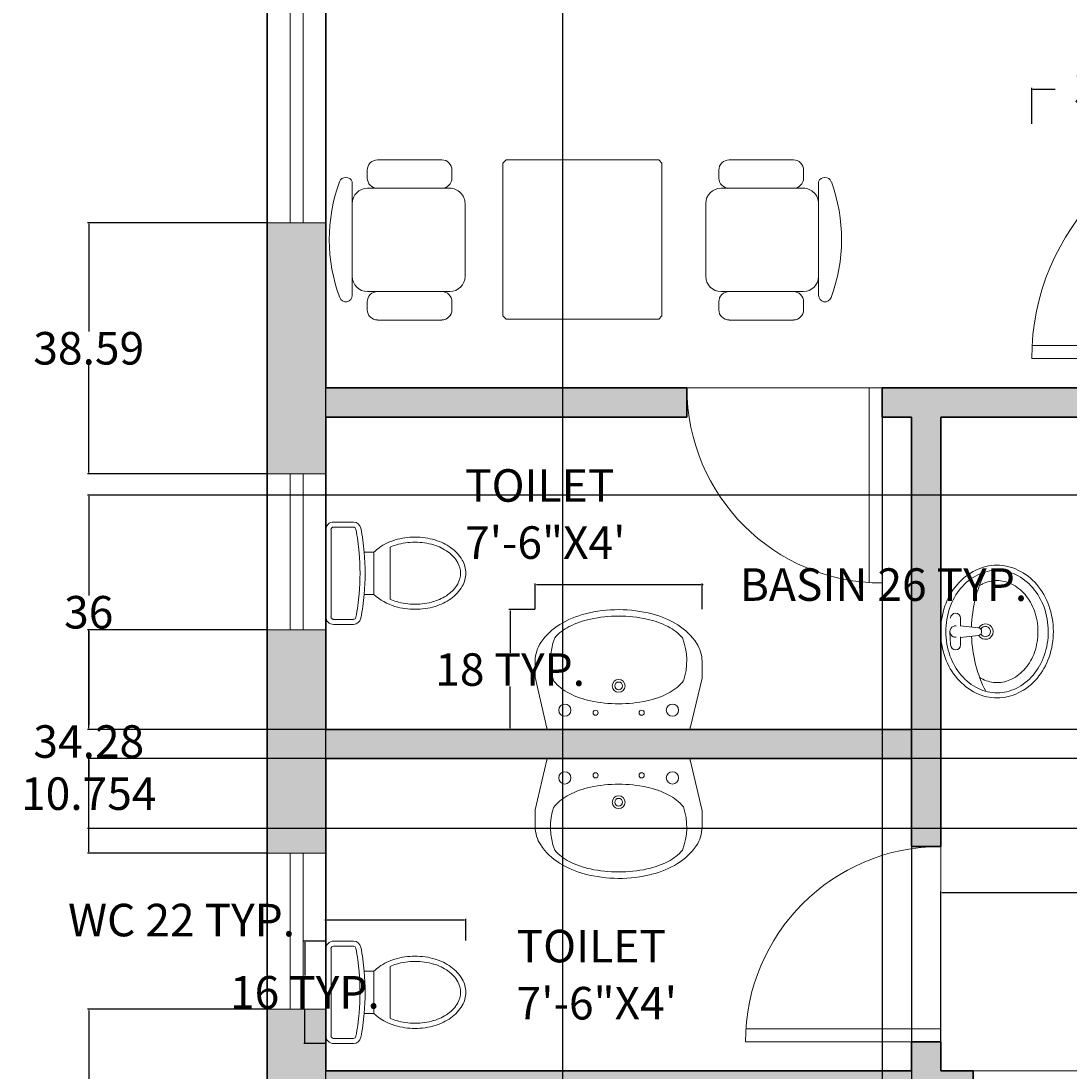
# Model space of a CAD drawing. Units: inches. Extents: x 2807 to 3326, y 2005 to 2580.
# Tile 8 of 12: x 2807 to 2968, y 2280 to 2441. Entities that reach past the tile are written whole.
import ezdxf

# ---------------------------------------------------------------- set-up
doc = ezdxf.new("R2010")
doc.units = ezdxf.units.IN
doc.header["$LTSCALE"] = 0.4
for name, color, linetype, lineweight in [('A-ANNO-DIMS', 2, 'Continuous', 18), ('A-AREA-IDEN', 5, 'Continuous', 18), ('A-FLOR-FIXT', 8, 'Continuous', 18), ('A-WALL-PATT', 231, 'Continuous', 13), ('DOORS', 144, 'Continuous', 18), ('Furniture', 7, 'Continuous', 15), ('WALL', 233, 'Continuous', 35), ('WINDOWS', 132, 'Continuous', 18)]:
    doc.layers.add(name, color=color, linetype=linetype, lineweight=lineweight)
doc.styles.get("Standard").update_dxf_attribs({"font": 'txt', "height": 5})
doc.dimstyles.get("Standard").update_dxf_attribs({"dimtxt": 0.18, "dimasz": 0.18, "dimexe": 0.18, "dimexo": 0.0625, "dimgap": 0.09, "dimtad": 0, "dimtih": 1, "dimtoh": 1, "dimdec": 4, "dimzin": 0, "dimdsep": 46, "dimtxsty": 'Standard', "dimcen": 0.09, "dimadec": 0, "dimazin": 0, "dimtfac": 1, "dimtdec": 4, "dimtofl": 0, "dimtmove": 0, "dimatfit": 3, "dimfxl": 1, "dimtolj": 1, "dimtzin": 0, "dimarcsym": 0})

# ---------------------------------------------------------------- blocks, each defined once
blk = doc.blocks.new('WIN-36')
at = {"ltscale": 0.4}
for p, q in [((0, 36), (0, 0)), ((9, 36), (0, 36)), ((3.5, 36), (3.5, 0)), ((5.5, 36), (5.5, 0)), ((9, 0), (9, 36)), ((0, 0), (9, 0))]:
    blk.add_line(p, q, dxfattribs=at)
blk = doc.blocks.new('WIN-24')
at = {"ltscale": 0.4}
for p, q in [((0, 0), (-9, 0)), ((-9, 0), (-9, -24)), ((-5.5, -24), (-5.5, 0)), ((-3.5, -24), (-3.5, 0)), ((0, -24), (0, 0)), ((-9, -24), (0, -24))]:
    blk.add_line(p, q, dxfattribs=at)
blk = doc.blocks.new('DOOR-30')
for p, q in [((0, 0), (-30, 0)), ((-2, -29.93), (-2, 0)), ((0, -30), (0, 0))]:
    blk.add_line(p, q)
blk.add_arc((0, 0), 30, 180, 270)
blk = doc.blocks.new('DOOR-36')
for p, q in [((0, 0), (-36, 0)), ((-2, -35.94), (-2, 0)), ((0, -36), (0, 0))]:
    blk.add_line(p, q)
blk.add_arc((0, 0), 36, 180, 270)
blk = doc.blocks.new('TABLE-SET-TWO')
for p, q in [((-7.94, 35.84), (-8.53, 35.84)), ((8.92, 35.84), (-7.94, 35.84)), ((-5.59, 35.84), (5.59, 35.84)), ((-10.73, 33.54), (-9.51, 33.54)), ((-7.94, 20.85), (-7.94, 33.49)), ((7.94, 33.49), (7.94, 20.85)), ((9.51, 33.54), (10.73, 33.54)), ((-12.31, 22.08), (-12.31, 31.97)), ((-7.94, 31.97), (-7.94, 22.08)), ((7.94, 22.08), (7.94, 31.97)), ((12.31, 31.97), (12.31, 22.08)), ((-9.51, 20.51), (-10.73, 20.51)), ((10.73, 20.51), (9.51, 20.51)), ((5.59, 18.5), (-5.59, 18.5)), ((-12.17, 12.19), (-11.66, 12.7)), ((-12.17, -11.26), (-12.17, 12.19)), ((-11.66, 12.7), (11.79, 12.7)), ((11.79, 12.7), (12.3, 12.19)), ((12.3, 12.19), (12.3, -11.26)), ((-11.66, -11.77), (-12.17, -11.26)), ((12.3, -11.26), (11.79, -11.77)), ((11.79, -11.77), (-11.66, -11.77)), ((5.59, -18.5), (-5.59, -18.5)), ((-9.51, -20.51), (-10.73, -20.51)), ((-7.94, -20.85), (-7.94, -33.49)), ((7.94, -33.49), (7.94, -20.85)), ((10.73, -20.51), (9.51, -20.51)), ((-12.31, -22.08), (-12.31, -31.97)), ((-7.94, -31.97), (-7.94, -22.08)), ((7.94, -22.08), (7.94, -31.97)), ((12.31, -31.97), (12.31, -22.08)), ((-10.73, -33.54), (-9.51, -33.54)), ((9.51, -33.54), (10.73, -33.54)), ((-7.94, -35.84), (-8.53, -35.84)), ((8.92, -35.84), (-7.94, -35.84)), ((-5.59, -35.84), (5.59, -35.84))]:
    blk.add_line(p, q)
for centre, radius, start, end in [((0.09, 13.6), 25.77, 69.9544, 110.3611), ((-8.53, 36.83), 0.986, 110.3611, 270), ((8.57, 36.82), 1.04, 290.0456, 69.9544), ((-5.59, 33.49), 2.35, 90, 180), ((5.59, 33.49), 2.35, 0, 90), ((-10.73, 31.97), 1.57, 90, 180), ((-9.51, 31.97), 1.57, 0, 90), ((9.51, 31.97), 1.57, 90, 180), ((10.73, 31.97), 1.57, 0, 90), ((-10.73, 22.08), 1.57, 180, 270), ((-9.51, 22.08), 1.57, 270, 0), ((9.51, 22.08), 1.57, 180, 270), ((10.73, 22.08), 1.57, 270, 0), ((-5.59, 20.85), 2.35, 180, 270), ((5.59, 20.85), 2.35, 270, 0), ((-5.59, -20.85), 2.35, 90, 180), ((5.59, -20.85), 2.35, 0, 90), ((-10.73, -22.08), 1.57, 90, 180), ((-9.51, -22.08), 1.57, 0, 90), ((9.51, -22.08), 1.57, 90, 180), ((10.73, -22.08), 1.57, 0, 90), ((-10.73, -31.97), 1.57, 180, 270), ((-9.51, -31.97), 1.57, 270, 0), ((9.51, -31.97), 1.57, 180, 270), ((10.73, -31.97), 1.57, 270, 0), ((-5.59, -33.49), 2.35, 180, 270), ((5.59, -33.49), 2.35, 270, 0), ((-8.53, -36.83), 0.986, 90, 249.6389), ((8.57, -36.82), 1.04, 290.0456, 69.9544), ((0.09, -13.6), 25.77, 249.6389, 290.0456)]:
    blk.add_arc(centre, radius, start, end)
blk = doc.blocks.new('WC')
for p, q in [((-1.18, 7.87), (-4.23, 7.87)), ((-1.18, 7.09), (-4.23, 7.09)), ((-0.79, -6.69), (-0.79, 6.69)), ((0, -6.69), (0, 6.69)), ((-9.87, -3.98), (-9.87, 3.98)), ((-7.37, -3.23), (-7.37, 3.26)), ((-7.37, 3.26), (-5.9, 3.26)), ((-7.37, -3.23), (-5.9, -3.23)), ((-4.23, -7.09), (-1.18, -7.09)), ((-4.23, -7.87), (-1.18, -7.87))]:
    blk.add_line(p, q)
for centre, radius, start, end in [((31.04, 0), 37.08, 169.2553, 174.96), ((-4.23, 6.69), 1.18, 90, 169.2553), ((31.04, 0), 36.29, 169.2553, 174.96), ((-4.23, 6.69), 0.394, 90, 169.2553), ((-1.18, 6.69), 1.18, 0, 90), ((-1.18, 6.69), 0.394, 0, 90), ((-14.49, -2.74), 8.17, 106.4045, 125.4032), ((-13.7, -5.39), 10.94, 90, 106.4045), ((-13.7, -5.39), 10.94, 73.5955, 90), ((-12.92, -2.74), 8.17, 47.2276, 73.5955), ((-15.68, -1.06), 6.11, 125.4032, 149.7669), ((-15.68, -1.06), 5.33, 125.4032, 149.7669), ((-14.49, -2.74), 7.39, 106.4045, 125.4032), ((-13.7, -5.39), 10.15, 90, 106.4045), ((-13.7, -5.39), 10.15, 73.5955, 90), ((-12.92, -2.74), 7.39, 65.5529, 73.5955), ((31.04, 0), 37.08, 174.96, 184.9899), ((-17.5, 0), 4, 149.7669, 180), ((-17.5, 0), 3.21, 149.7669, 180), ((31.04, 0), 36.29, 174.96, 184.9899), ((-17.5, 0), 4, 180, 210.2331), ((-17.5, 0), 3.21, 180, 210.2331), ((-15.68, 1.06), 6.11, 210.2331, 234.5968), ((-15.68, 1.06), 5.33, 210.2331, 234.5968), ((-11.73, 1.06), 6.11, 305.4032, 315.4553), ((31.04, 0), 37.08, 184.9899, 190.7447), ((31.04, 0), 36.29, 184.9899, 190.7447), ((-14.49, 2.74), 8.17, 234.5968, 253.5955), ((-14.49, 2.74), 7.39, 234.5968, 253.5955), ((-13.7, 5.39), 10.15, 253.5955, 270), ((-13.7, 5.39), 10.15, 270, 286.4045), ((-12.92, 2.74), 7.39, 286.4045, 294.4471), ((-12.92, 2.74), 8.17, 286.4045, 305.4032), ((-13.7, 5.39), 10.94, 253.5955, 270), ((-13.7, 5.39), 10.94, 270, 286.4045), ((-4.23, -6.69), 1.18, 190.7447, 270), ((-4.23, -6.69), 0.394, 190.7447, 270), ((-1.18, -6.69), 0.394, 270, 0), ((-1.18, -6.69), 1.18, 270, 0)]:
    blk.add_arc(centre, radius, start, end)
blk = doc.blocks.new('LAVATORY-WALL')
for p, q in [((-12.82, 8.02), (-12.82, 10.56)), ((12.82, 8.02), (12.82, 10.56)), ((-12.82, 8.02), (-11.02, 0.2)), ((9.76, 7.2), (9.85, 7.28)), ((9.86, 7.44), (9.86, 7.31)), ((12.82, 7.85), (11.02, 0.2)), ((-11.02, 0), (-11.02, 0.39)), ((11.02, 0), (-11.02, 0)), ((11.02, 0.39), (11.02, 0))]:
    blk.add_line(p, q)
for centre, radius in [((0, 6.69), 0.984), ((0, 6.69), 0.591), ((-8.27, 2.95), 0.945), ((8.27, 2.95), 0.945), ((8.27, 2.95), 0.945), ((8.27, 2.95), 0.945), ((-3.54, 2.56), 0.394), ((3.54, 2.56), 0.394)]:
    blk.add_circle(centre, radius)
for centre, radius, start, end in [((-1.65, 3.98), 14.22, 104.0583, 121.3573), ((-0.05, -2.38), 20.78, 89.7676, 104.0583), ((-0.05, -2.38), 20.78, 75.477, 89.7676), ((-1.62, 4.13), 13.11, 102.0046, 117.1742), ((0, -3.48), 20.89, 90, 102.0046), ((0, -3.48), 20.89, 77.9954, 90), ((1.62, 4.13), 13.11, 62.8258, 77.9954), ((1.59, 3.97), 14.22, 58.1779, 75.477), ((-4.1, 8.01), 9.5, 121.3573, 145.8048), ((-4.07, 8.92), 7.73, 117.1742, 138.1444), ((4.07, 8.92), 7.73, 41.9499, 62.8258), ((4.08, 7.98), 9.5, 33.7305, 58.1779), ((-7.83, 10.54), 4.99, 145.8048, 179.7676), ((-0.53, 10.56), 9.94, 159.3022, 198.4613), ((0.53, 10.56), 9.94, 341.5387, 20.6978), ((7.83, 10.48), 4.99, 359.7676, 33.7305), ((-7.83, 10.54), 4.99, 179.7676, 180.9606), ((-4.07, 12.42), 7.73, 220.3901, 242.8258), ((4.07, 12.42), 7.73, 297.1742, 318.6261), ((9.82, 7.31), 0.0394, 311.3224, 0), ((7.83, 8.04), 4.99, 357.883, 359.7676), ((-1.62, 17.21), 13.11, 242.8258, 257.9954), ((1.62, 17.21), 13.11, 282.0046, 297.1742), ((0, 24.82), 20.89, 257.9954, 270), ((0, 24.82), 20.89, 270, 282.0046)]:
    blk.add_arc(centre, radius, start, end)
at = {"width": 0.8, "flags": 9}
for tag in ['XSIZE', 'YSIZE']:
    blk.add_attdef(tag, (0, 0), '', height=0.0197, rotation=180, dxfattribs=at)
blk = doc.blocks.new('*D18')
at = {"layer": 'A-ANNO-DIMS', "color": 0, "lineweight": -2, "ltscale": 0.4, "transparency": 16777216}
for p, q in [((2962.07, 2425.14), (2962.07, 2430.66)), ((2962.25, 2430.48), (2965.69, 2430.48)), ((2997.89, 2430.48), (2994.44, 2430.48)), ((2998.07, 2425.14), (2998.07, 2430.66))]:
    blk.add_line(p, q, dxfattribs=at)
at = {"layer": 'A-ANNO-DIMS', "color": 0, "ltscale": 0.4, "transparency": 16777216}
for points in [[(2962.25, 2430.51), (2962.25, 2430.45), (2962.07, 2430.48)], [(2997.89, 2430.51), (2997.89, 2430.45), (2998.07, 2430.48)]]:
    blk.add_solid(points, dxfattribs=at)
at = {"layer": 'Defpoints', "color": 0, "ltscale": 0.4, "transparency": 16777216}
for p in [(2998.07, 2430.48), (2962.07, 2425.08), (2998.07, 2425.08)]:
    blk.add_point(p, dxfattribs=at)
at = {"layer": 'A-ANNO-DIMS', "color": 0, "ltscale": 0.4, "transparency": 16777216, "insert": (2980.07, 2430.48), "char_height": 5, "attachment_point": 5}
blk.add_mtext('\\A1;36 TYP.', dxfattribs=at)
blk = doc.blocks.new('*D23')
at = {"layer": 'A-ANNO-DIMS', "color": 0, "lineweight": -2, "ltscale": 0.4, "transparency": 16777216}
for p, q in [((2853.57, 2302.77), (2853.39, 2302.77)), ((2853.57, 2299.61), (2853.57, 2302.95)), ((2874.89, 2302.77), (2853.75, 2302.77)), ((2875.07, 2299.61), (2875.07, 2302.95))]:
    blk.add_line(p, q, dxfattribs=at)
at = {"layer": 'A-ANNO-DIMS', "color": 0, "ltscale": 0.4, "transparency": 16777216}
for points in [[(2853.75, 2302.8), (2853.75, 2302.74), (2853.57, 2302.77)], [(2874.89, 2302.8), (2874.89, 2302.74), (2875.07, 2302.77)]]:
    blk.add_solid(points, dxfattribs=at)
at = {"layer": 'Defpoints', "color": 0, "ltscale": 0.4, "transparency": 16777216}
for p in [(2853.57, 2302.77), (2853.57, 2299.54), (2875.07, 2299.54)]:
    blk.add_point(p, dxfattribs=at)
at = {"layer": 'A-ANNO-DIMS', "color": 0, "ltscale": 0.4, "transparency": 16777216, "insert": (2831.39, 2302.77), "char_height": 5, "attachment_point": 5}
blk.add_mtext('\\A1;WC 22 TYP.', dxfattribs=at)
blk = doc.blocks.new('*D24')
at = {"layer": 'A-ANNO-DIMS', "color": 0, "lineweight": -2, "ltscale": 0.4, "transparency": 16777216}
for p, q in [((2853.5, 2299.54), (2850.16, 2299.54)), ((2850.34, 2299.36), (2850.34, 2294.26)), ((2850.34, 2283.98), (2850.34, 2289.08)), ((2853.5, 2283.8), (2850.16, 2283.8))]:
    blk.add_line(p, q, dxfattribs=at)
at = {"layer": 'A-ANNO-DIMS', "color": 0, "ltscale": 0.4, "transparency": 16777216}
for points in [[(2850.31, 2299.36), (2850.37, 2299.36), (2850.34, 2299.54)], [(2850.31, 2283.98), (2850.37, 2283.98), (2850.34, 2283.8)]]:
    blk.add_solid(points, dxfattribs=at)
at = {"layer": 'Defpoints', "color": 0, "ltscale": 0.4, "transparency": 16777216}
for p in [(2853.57, 2299.54), (2850.34, 2283.8), (2853.57, 2283.8)]:
    blk.add_point(p, dxfattribs=at)
at = {"layer": 'A-ANNO-DIMS', "color": 0, "ltscale": 0.4, "transparency": 16777216, "insert": (2850.34, 2291.67), "char_height": 5, "attachment_point": 5}
blk.add_mtext('\\A1;16 TYP.', dxfattribs=at)
blk = doc.blocks.new('*D25')
at = {"layer": 'A-ANNO-DIMS', "color": 0, "lineweight": -2, "ltscale": 0.4, "transparency": 16777216}
for p, q in [((2885.74, 2350.54), (2885.74, 2354.51)), ((2885.92, 2354.33), (2911.22, 2354.33)), ((2911.4, 2350.54), (2911.4, 2354.51)), ((2911.4, 2354.33), (2911.58, 2354.33))]:
    blk.add_line(p, q, dxfattribs=at)
at = {"layer": 'A-ANNO-DIMS', "color": 0, "ltscale": 0.4, "transparency": 16777216}
for points in [[(2885.92, 2354.36), (2885.92, 2354.3), (2885.74, 2354.33)], [(2911.22, 2354.36), (2911.22, 2354.3), (2911.4, 2354.33)]]:
    blk.add_solid(points, dxfattribs=at)
at = {"layer": 'Defpoints', "color": 0, "ltscale": 0.4, "transparency": 16777216}
for p in [(2911.4, 2354.33), (2885.74, 2350.48), (2911.4, 2350.48)]:
    blk.add_point(p, dxfattribs=at)
at = {"layer": 'A-ANNO-DIMS', "color": 0, "ltscale": 0.4, "transparency": 16777216, "insert": (2939.28, 2354.33), "char_height": 5, "attachment_point": 5}
blk.add_mtext('\\A1;BASIN 26 TYP.', dxfattribs=at)
blk = doc.blocks.new('*D26')
at = {"layer": 'A-ANNO-DIMS', "color": 0, "lineweight": -2, "ltscale": 0.4, "transparency": 16777216}
for p, q in [((2885.68, 2350.48), (2881.71, 2350.48)), ((2881.89, 2350.3), (2881.89, 2343.86)), ((2881.89, 2332.24), (2881.89, 2338.68)), ((2885.68, 2332.06), (2881.71, 2332.06))]:
    blk.add_line(p, q, dxfattribs=at)
at = {"layer": 'A-ANNO-DIMS', "color": 0, "ltscale": 0.4, "transparency": 16777216}
for points in [[(2881.86, 2350.3), (2881.92, 2350.3), (2881.89, 2350.48)], [(2881.86, 2332.24), (2881.92, 2332.24), (2881.89, 2332.06)]]:
    blk.add_solid(points, dxfattribs=at)
at = {"layer": 'Defpoints', "color": 0, "ltscale": 0.4, "transparency": 16777216}
for p in [(2881.89, 2350.48), (2885.74, 2350.48), (2885.74, 2332.06)]:
    blk.add_point(p, dxfattribs=at)
at = {"layer": 'A-ANNO-DIMS', "color": 0, "ltscale": 0.4, "transparency": 16777216, "insert": (2881.89, 2341.27), "char_height": 5, "attachment_point": 5}
blk.add_mtext('\\A1;18 TYP.', dxfattribs=at)
blk = doc.blocks.new('*D37')
at = {"layer": 'A-ANNO-DIMS', "color": 0, "lineweight": -2, "ltscale": 0.4, "transparency": 16777216}
for p, q in [((2853.567191, 2144.638996), (2853.567191, 2577.206496)), ((2853.747191, 2577.026496), (2859.189306, 2577.026496)), ((2889.811421, 2577.026496), (2884.369306, 2577.026496)), ((2889.991421, 2144.638996), (2889.991421, 2577.206496))]:
    blk.add_line(p, q, dxfattribs=at)
at = {"layer": 'A-ANNO-DIMS', "color": 0, "ltscale": 0.4, "transparency": 16777216}
for points in [[(2853.747191, 2577.056496), (2853.747191, 2576.996496), (2853.567191, 2577.026496)], [(2889.811421, 2577.056496), (2889.811421, 2576.996496), (2889.991421, 2577.026496)]]:
    blk.add_solid(points, dxfattribs=at)
at = {"layer": 'Defpoints', "color": 0, "ltscale": 0.4, "transparency": 16777216}
for p in [(2889.991421, 2577.026496), (2853.567191, 2144.576496), (2889.991421, 2144.576496)]:
    blk.add_point(p, dxfattribs=at)
at = {"layer": 'A-ANNO-DIMS', "color": 0, "ltscale": 0.4, "transparency": 16777216, "insert": (2871.779306, 2577.026496), "char_height": 5, "attachment_point": 5}
blk.add_mtext('\\A1;36.424', dxfattribs=at)
blk = doc.blocks.new('*D42')
at = {"layer": 'A-ANNO-DIMS', "color": 0, "lineweight": -2, "ltscale": 0.4, "transparency": 16777216}
for p, q in [((2844.504691, 2289.066335), (2816.937191, 2289.066335)), ((2817.117191, 2288.886335), (2817.117191, 2261.071202)), ((2817.117191, 2228.076069), (2817.117191, 2255.891202)), ((2844.504691, 2227.896069), (2816.937191, 2227.896069))]:
    blk.add_line(p, q, dxfattribs=at)
at = {"layer": 'A-ANNO-DIMS', "color": 0, "ltscale": 0.4, "transparency": 16777216}
for points in [[(2817.087191, 2288.886335), (2817.147191, 2288.886335), (2817.117191, 2289.066335)], [(2817.087191, 2228.076069), (2817.147191, 2228.076069), (2817.117191, 2227.896069)]]:
    blk.add_solid(points, dxfattribs=at)
at = {"layer": 'Defpoints', "color": 0, "ltscale": 0.4, "transparency": 16777216}
for p in [(2817.117191, 2289.066335), (2844.567191, 2289.066335), (2844.567191, 2227.896069)]:
    blk.add_point(p, dxfattribs=at)
at = {"layer": 'A-ANNO-DIMS', "color": 0, "ltscale": 0.4, "transparency": 16777216, "insert": (2817.117191, 2258.481202), "char_height": 5, "attachment_point": 5}
blk.add_mtext('\\A1;61.17', dxfattribs=at)
blk = doc.blocks.new('*D43')
at = {"layer": 'A-ANNO-DIMS', "color": 0, "lineweight": -2, "ltscale": 0.4, "transparency": 16777216}
for p, q in [((2844.5, 2347.35), (2816.94, 2347.35)), ((2817.12, 2347.17), (2817.12, 2332.8)), ((2817.12, 2313.25), (2817.12, 2327.62)), ((2844.5, 2313.07), (2816.94, 2313.07))]:
    blk.add_line(p, q, dxfattribs=at)
at = {"layer": 'A-ANNO-DIMS', "color": 0, "ltscale": 0.4, "transparency": 16777216}
for points in [[(2817.09, 2347.17), (2817.15, 2347.17), (2817.12, 2347.35)], [(2817.09, 2313.25), (2817.15, 2313.25), (2817.12, 2313.07)]]:
    blk.add_solid(points, dxfattribs=at)
at = {"layer": 'Defpoints', "color": 0, "ltscale": 0.4, "transparency": 16777216}
for p in [(2817.12, 2347.35), (2844.57, 2347.35), (2844.57, 2313.07)]:
    blk.add_point(p, dxfattribs=at)
at = {"layer": 'A-ANNO-DIMS', "color": 0, "ltscale": 0.4, "transparency": 16777216, "insert": (2817.12, 2330.21), "char_height": 5, "attachment_point": 5}
blk.add_mtext('\\A1;34.28', dxfattribs=at)
blk = doc.blocks.new('*D44')
at = {"layer": 'A-ANNO-DIMS', "color": 0, "lineweight": -2, "ltscale": 0.4, "transparency": 16777216}
for p, q in [((2844.504691, 2409.939958), (2816.937191, 2409.939958)), ((2817.117191, 2409.759958), (2817.117191, 2393.234837)), ((2817.117191, 2371.529716), (2817.117191, 2388.054837)), ((2844.504691, 2371.349716), (2816.937191, 2371.349716))]:
    blk.add_line(p, q, dxfattribs=at)
at = {"layer": 'A-ANNO-DIMS', "color": 0, "ltscale": 0.4, "transparency": 16777216}
for points in [[(2817.087191, 2409.759958), (2817.147191, 2409.759958), (2817.117191, 2409.939958)], [(2817.087191, 2371.529716), (2817.147191, 2371.529716), (2817.117191, 2371.349716)]]:
    blk.add_solid(points, dxfattribs=at)
at = {"layer": 'Defpoints', "color": 0, "ltscale": 0.4, "transparency": 16777216}
for p in [(2817.117191, 2409.939958), (2844.567191, 2409.939958), (2844.567191, 2371.349716)]:
    blk.add_point(p, dxfattribs=at)
at = {"layer": 'A-ANNO-DIMS', "color": 0, "ltscale": 0.4, "transparency": 16777216, "insert": (2817.117191, 2390.644837), "char_height": 5, "attachment_point": 5}
blk.add_mtext('\\A1;38.59', dxfattribs=at)
blk = doc.blocks.new('*D46')
at = {"layer": 'A-ANNO-DIMS', "color": 0, "lineweight": -2, "ltscale": 0.4, "transparency": 16777216}
for p, q in [((3279.5, 2327.58), (2816.94, 2327.58)), ((2817.12, 2327.4), (2817.12, 2324.79)), ((2817.12, 2317), (2817.12, 2319.61)), ((3279.5, 2316.82), (2816.94, 2316.82))]:
    blk.add_line(p, q, dxfattribs=at)
at = {"layer": 'A-ANNO-DIMS', "color": 0, "ltscale": 0.4, "transparency": 16777216}
for points in [[(2817.09, 2327.4), (2817.15, 2327.4), (2817.12, 2327.58)], [(2817.09, 2317), (2817.15, 2317), (2817.12, 2316.82)]]:
    blk.add_solid(points, dxfattribs=at)
at = {"layer": 'Defpoints', "color": 0, "ltscale": 0.4, "transparency": 16777216}
for p in [(2817.12, 2327.58), (3279.57, 2327.58), (3279.57, 2316.82)]:
    blk.add_point(p, dxfattribs=at)
at = {"layer": 'A-ANNO-DIMS', "color": 0, "ltscale": 0.4, "transparency": 16777216, "insert": (2817.12, 2322.2), "char_height": 5, "attachment_point": 5}
blk.add_mtext('\\A1;10.754', dxfattribs=at)
blk = doc.blocks.new('*D47')
at = {"layer": 'A-ANNO-DIMS', "color": 0, "lineweight": -2, "ltscale": 0.4, "transparency": 16777216}
for p, q in [((3279.504691, 2368.076496), (2816.937191, 2368.076496)), ((2817.117191, 2367.896496), (2817.117191, 2352.666496)), ((2817.117191, 2332.256496), (2817.117191, 2347.486496)), ((3279.504691, 2332.076496), (2816.937191, 2332.076496))]:
    blk.add_line(p, q, dxfattribs=at)
at = {"layer": 'A-ANNO-DIMS', "color": 0, "ltscale": 0.4, "transparency": 16777216}
for points in [[(2817.087191, 2367.896496), (2817.147191, 2367.896496), (2817.117191, 2368.076496)], [(2817.087191, 2332.256496), (2817.147191, 2332.256496), (2817.117191, 2332.076496)]]:
    blk.add_solid(points, dxfattribs=at)
at = {"layer": 'Defpoints', "color": 0, "ltscale": 0.4, "transparency": 16777216}
for p in [(2817.117191, 2368.076496), (3279.567191, 2368.076496), (3279.567191, 2332.076496)]:
    blk.add_point(p, dxfattribs=at)
at = {"layer": 'A-ANNO-DIMS', "color": 0, "ltscale": 0.4, "transparency": 16777216, "insert": (2817.117191, 2350.076496), "char_height": 5, "attachment_point": 5}
blk.add_mtext('\\A1;36', dxfattribs=at)
blk = doc.blocks.new('*D69')
at = {"layer": 'A-ANNO-DIMS', "color": 0, "lineweight": -2, "ltscale": 0.4, "transparency": 16777216}
for p, q in [((2939.07, 2380.01), (2939.07, 2008.45)), ((2943.57, 2380.01), (2943.57, 2008.45)), ((2939.25, 2008.63), (2943.39, 2008.63)), ((2943.57, 2008.63), (2943.75, 2008.63))]:
    blk.add_line(p, q, dxfattribs=at)
at = {"layer": 'A-ANNO-DIMS', "color": 0, "ltscale": 0.4, "transparency": 16777216}
for points in [[(2939.25, 2008.66), (2939.25, 2008.6), (2939.07, 2008.63)], [(2943.39, 2008.66), (2943.39, 2008.6), (2943.57, 2008.63)]]:
    blk.add_solid(points, dxfattribs=at)
at = {"layer": 'Defpoints', "color": 0, "ltscale": 0.4, "transparency": 16777216}
for p in [(2939.07, 2380.08), (2943.57, 2380.08), (2943.57, 2008.63)]:
    blk.add_point(p, dxfattribs=at)
at = {"layer": 'A-ANNO-DIMS', "color": 0, "ltscale": 0.4, "transparency": 16777216, "insert": (2949.08, 2008.63), "char_height": 5, "attachment_point": 5}
blk.add_mtext('\\A1;4.5', dxfattribs=at)
blk = doc.blocks.new('*D72')
at = {"layer": 'A-ANNO-DIMS', "color": 0, "lineweight": -2, "ltscale": 0.4, "transparency": 16777216}
for p, q in [((2948.07, 2279.64), (2948.07, 2307.21)), ((2948.25, 2307.03), (3060.05, 2307.03)), ((3184.89, 2307.03), (3073.09, 2307.03)), ((3185.07, 2279.64), (3185.07, 2307.21))]:
    blk.add_line(p, q, dxfattribs=at)
at = {"layer": 'A-ANNO-DIMS', "color": 0, "ltscale": 0.4, "transparency": 16777216}
for points in [[(2948.25, 2307.06), (2948.25, 2307), (2948.07, 2307.03)], [(3184.89, 2307.06), (3184.89, 2307), (3185.07, 2307.03)]]:
    blk.add_solid(points, dxfattribs=at)
at = {"layer": 'Defpoints', "color": 0, "ltscale": 0.4, "transparency": 16777216}
for p in [(3185.07, 2307.03), (2948.07, 2279.58), (3185.07, 2279.58)]:
    blk.add_point(p, dxfattribs=at)
at = {"layer": 'A-ANNO-DIMS', "color": 0, "ltscale": 0.4, "transparency": 16777216, "insert": (3066.57, 2307.03), "char_height": 5, "attachment_point": 5}
blk.add_mtext('\\A1;237', dxfattribs=at)

msp = doc.modelspace()

# ---------------------------------------------------------------- hatches: boundary and pattern name
at = {"layer": 'A-WALL-PATT', "ltscale": 0.4}
h = msp.add_hatch(color=256, dxfattribs=at)
h.dxf.hatch_style = 1
h.paths.add_polyline_path([(3288.5672, 2549.5765), (2941.5672, 2549.5765), (2941.5672, 2540.5765), (2993.5672, 2540.5765), (2993.5672, 2489.5693), (2998.0672, 2489.5693), (2998.0672, 2540.5765), (3135.0672, 2540.5765), (3135.0672, 2479.0765), (3139.5672, 2479.0765), (3139.5672, 2540.5765), (3279.5672, 2540.5765), (3279.5672, 2510.5765), (3288.5672, 2510.5765)])
h.paths.add_polyline_path([(2905.5672, 2549.5765), (2844.5672, 2549.5765), (2844.5672, 2445.94), (2853.5672, 2445.94), (2853.5672, 2540.5765), (2905.5672, 2540.5765)])
h.paths.add_polyline_path([(2853.5672, 2409.94), (2844.5672, 2409.94), (2844.5672, 2371.3497), (2853.5672, 2371.3497), (2853.5672, 2380.0765), (2909.0672, 2380.0765), (2909.0672, 2384.5765), (2853.5672, 2384.5765)])
h.paths.add_polyline_path([(2998.0672, 2389.0765), (2993.5672, 2389.0765), (2993.5672, 2384.5765), (2939.0672, 2384.5765), (2939.0672, 2380.0765), (2943.5672, 2380.0765), (2943.5672, 2314.0765), (2948.0672, 2314.0765), (2948.0672, 2380.0765), (2998.0672, 2380.0765)])
h.paths.add_polyline_path([(2998.0672, 2471.8029), (2993.5672, 2471.8029), (2993.5672, 2425.0765), (2998.0672, 2425.0765)])
h.paths.add_polyline_path([(2953.0672, 2279.5765), (2948.0672, 2279.5765), (2948.0672, 2284.0765), (2943.5672, 2284.0765), (2943.5672, 2279.5765), (2853.5672, 2279.5765), (2853.5672, 2289.0663), (2844.5672, 2289.0663), (2844.5672, 2227.8961), (2853.5672, 2227.8961), (2853.5672, 2275.0765), (2953.0672, 2275.0765)])
h.paths.add_polyline_path([(2943.5672, 2332.0765), (2853.5672, 2332.0765), (2853.5672, 2347.3497), (2844.5672, 2347.3497), (2844.5672, 2313.0663), (2853.5672, 2313.0663), (2853.5672, 2327.5765), (2943.5672, 2327.5765)])
h.paths.add_polyline_path([(3144.0672, 2279.5765), (2993.5672, 2279.5765), (2989.0672, 2279.5765), (2989.0672, 2275.0765), (2993.5672, 2275.0765), (2993.5672, 2144.5765), (2984.5672, 2144.5765), (2984.5672, 2135.5765), (2993.5672, 2135.5765), (2993.5672, 2120.0765), (3036.5672, 2120.0765), (3036.5672, 2129.0765), (2998.0672, 2129.0765), (2998.0672, 2275.0765), (3135.0672, 2275.0765), (3135.0672, 2129.0765), (3096.5672, 2129.0765), (3096.5672, 2120.0765), (3139.5672, 2120.0765), (3139.5672, 2135.5765), (3148.5672, 2135.5765), (3148.5672, 2144.5765), (3139.5672, 2144.5765), (3139.5672, 2275.0765), (3144.0672, 2275.0765)])
h.paths.add_polyline_path([(2984.5672, 2144.5765), (2925.9914, 2144.5765), (2925.9914, 2135.5765), (2984.5672, 2135.5765)])
h.paths.add_polyline_path([(2889.9914, 2144.5765), (2853.5672, 2144.5765), (2853.5672, 2191.8961), (2844.5672, 2191.8961), (2844.5672, 2135.5765), (2889.9914, 2135.5765)])
h.paths.add_polyline_path([(3196.0672, 2144.5765), (3148.5672, 2144.5765), (3148.5672, 2135.5765), (3196.0672, 2135.5765)])
h.paths.add_polyline_path([(3288.5672, 2191.8265), (3279.5672, 2191.8265), (3279.5672, 2144.5765), (3232.0672, 2144.5765), (3232.0672, 2135.5765), (3288.5672, 2135.5765)])
h.paths.add_polyline_path([(3288.5672, 2292.8229), (3279.5672, 2292.8229), (3279.5672, 2291.4371), (3279.5672, 2279.5765), (3189.5672, 2279.5765), (3189.5672, 2293.0765), (3185.0672, 2293.0765), (3185.0672, 2279.5765), (3180.0672, 2279.5765), (3180.0672, 2275.0765), (3279.5672, 2275.0765), (3279.5672, 2227.8265), (3288.5672, 2227.8265)])
h.paths.add_polyline_path([(3288.5672, 2368.0765), (3279.5672, 2368.0765), (3279.5672, 2332.0765), (3174.0672, 2332.0765), (3174.0672, 2327.5765), (3185.0672, 2327.5765), (3189.5672, 2327.5765), (3279.5672, 2327.5765), (3279.5672, 2316.8229), (3288.5672, 2316.8229)])
h.paths.add_polyline_path([(3288.5672, 2474.5765), (3279.5672, 2474.5765), (3279.5672, 2444.5765), (3139.5672, 2444.5765), (3139.5672, 2449.0765), (3135.0672, 2449.0765), (3135.0672, 2327.5765), (3144.0672, 2327.5765), (3144.0672, 2332.0765), (3139.5672, 2332.0765), (3139.5672, 2440.0765), (3279.5672, 2440.0765), (3279.5672, 2404.0765), (3288.5672, 2404.0765)])

# ---------------------------------------------------------------- linework, layer by layer
at = {"layer": 'A-FLOR-FIXT'}
for p, q in [((2951.1113, 2347.9678), (2953.8682, 2347.682)), ((2951.1236, 2349.1572), (2951.1279, 2347.9187)), ((2949.6023, 2345.0575), (2949.4771, 2347.1043)), ((2951.1173, 2346.2062), (2953.8722, 2346.5109)), ((2951.1377, 2345.0628), (2951.1334, 2346.3014))]:
    msp.add_line(p, q, dxfattribs=at)
for centre, radius, start, end in [((2957.384, 2348.5555), 8.9023, 116.192801, 139.851712), ((2973.2805, 2347.1632), 20.4891, 153.617787, 178.239687), ((2956.7189, 2349.9076), 7.3955, 90.196979, 116.192801), ((2956.7189, 2349.9076), 6.6081, 90.196979, 116.192801), ((2956.7189, 2349.9076), 7.3955, 64.201156, 90.196979), ((2956.7189, 2349.9076), 6.6081, 64.201156, 90.196979), ((2956.0631, 2348.5509), 8.9023, 40.542245, 64.201156), ((2958.4193, 2347.6822), 10.2568, 139.851712, 160.812984), ((2957.384, 2348.5555), 8.1149, 116.192801, 139.851712), ((2957.384, 2348.5555), 6.5401, 116.192801, 120.894354), ((2956.7189, 2349.9076), 5.0333, 90.196979, 116.192801), ((2956.7189, 2349.9076), 5.0333, 64.201156, 90.196979), ((2956.0631, 2348.5509), 6.5401, 40.542245, 64.201156), ((2956.0631, 2348.5509), 8.1149, 40.542245, 64.201156), ((2955.0339, 2347.6706), 10.2568, 19.580973, 40.542245), ((2958.4193, 2347.6822), 9.4694, 139.851712, 160.812984), ((2955.0339, 2347.6706), 7.8946, 19.580974, 40.542245), ((2955.0339, 2347.6706), 9.4694, 19.580974, 40.542245), ((2953.4155, 2347.0949), 11.9745, 0.196979, 19.580973), ((2960.0416, 2347.1177), 11.9745, 160.812984, 180.196979), ((2960.0416, 2347.1177), 11.1871, 160.812984, 180.196979), ((2950.3559, 2349.1546), 0.7677, 0.196979, 180.196979), ((2953.4155, 2347.0949), 9.6123, 0.196979, 19.580973), ((2953.4155, 2347.0949), 11.1871, 0.196979, 19.580973), ((2950.363, 2347.1074), 0.8858, 84.081475, 276.312482), ((2954.9569, 2347.1002), 1.1811, 209.152003, 151.241954), ((2954.9569, 2347.1002), 0.7874, 206.581308, 153.812649), ((2960.0416, 2347.1177), 11.9745, 180.196979, 199.580973), ((2960.0416, 2347.1177), 11.1871, 180.196979, 199.580973), ((2973.2805, 2347.1632), 20.4891, 182.15427, 206.77617), ((2953.7758, 2347.0961), 0.5906, 279.392248, 81.001709), ((2953.4155, 2347.0949), 9.6123, 340.812984, 0.196979), ((2953.4155, 2347.0949), 11.1871, 340.812984, 0.196979), ((2953.4155, 2347.0949), 11.9745, 340.812984, 0.196979), ((2950.37, 2345.0601), 0.7677, 180.196979, 0.196979), ((2958.4232, 2346.542), 10.2568, 199.580973, 220.542245), ((2958.4232, 2346.542), 9.4694, 199.580973, 220.542245), ((2955.0378, 2346.5304), 7.8946, 319.851712, 340.812984), ((2955.0378, 2346.5304), 9.4694, 319.851712, 340.812984), ((2955.0378, 2346.5304), 10.2568, 319.851712, 340.812984), ((2956.0731, 2345.6571), 6.5401, 296.192801, 319.851712), ((2957.3939, 2345.6616), 8.9023, 220.542245, 244.201156), ((2957.3939, 2345.6616), 8.1149, 220.542245, 244.201156), ((2957.3939, 2345.6616), 6.5401, 239.499603, 244.201156), ((2956.7382, 2344.305), 5.0333, 244.201156, 270.196979), ((2956.7382, 2344.305), 5.0333, 270.196979, 296.192801), ((2956.0731, 2345.6571), 8.1149, 296.192801, 319.851712), ((2956.0731, 2345.6571), 8.9023, 296.192801, 319.851712), ((2956.7382, 2344.305), 6.6081, 244.201156, 270.196979), ((2956.7382, 2344.305), 6.6081, 270.196979, 296.192801), ((2956.7382, 2344.305), 7.3955, 244.201156, 270.196979), ((2956.7382, 2344.305), 7.3955, 270.196979, 296.192801)]:
    msp.add_arc(centre, radius, start, end, dxfattribs=at)
at = {"layer": 'WALL'}
for p, q in [((2844.5672, 2135.5765), (2844.5672, 2549.5765)), ((2853.5672, 2384.5765), (2853.5672, 2540.5765)), ((2853.5672, 2384.5765), (2909.0672, 2384.5765)), ((2909.0672, 2380.0765), (2909.0672, 2384.5765)), ((2939.0672, 2380.0765), (2939.0672, 2384.5765)), ((2939.0672, 2384.5765), (2993.5672, 2384.5765)), ((2853.5672, 2380.0765), (2909.0672, 2380.0765)), ((2853.5672, 2332.0765), (2853.5672, 2380.0765)), ((2939.0672, 2380.0765), (2943.5672, 2380.0765)), ((2943.5672, 2314.0765), (2943.5672, 2380.0765)), ((2948.0672, 2380.0765), (2998.0672, 2380.0765)), ((2948.0672, 2314.0765), (2948.0672, 2380.0765)), ((2853.5672, 2332.0765), (2943.5672, 2332.0765)), ((2853.5672, 2327.5765), (2943.5672, 2327.5765)), ((2853.5672, 2279.5765), (2853.5672, 2327.5765)), ((2943.5672, 2314.0765), (2948.0672, 2314.0765)), ((2943.5672, 2279.5765), (2943.5672, 2284.0765)), ((2943.5672, 2284.0765), (2948.0672, 2284.0765)), ((2948.0672, 2279.5765), (2948.0672, 2284.0765)), ((2853.5672, 2279.5765), (2943.5672, 2279.5765)), ((2948.0672, 2279.5765), (2953.0672, 2279.5765)), ((2953.0672, 2275.0765), (2953.0672, 2279.5765))]:
    msp.add_line(p, q, dxfattribs=at)

# ---------------------------------------------------------------- block references
at = {"layer": 'A-FLOR-FIXT', "rotation": 180}
for name, p in [('WC', (2853.5674, 2356.0764)), ('LAVATORY-WALL', (2898.5672, 2327.5765)), ('WC', (2853.5674, 2291.67))]:
    msp.add_blockref(name, p, dxfattribs=at)
at = {"layer": 'A-FLOR-FIXT'}
msp.add_blockref('LAVATORY-WALL', (2898.5672, 2332.0765), dxfattribs=at)
at = {"layer": 'DOORS'}
for name, p, rotation in [('DOOR-36', (2998.0672, 2389.0765), 269.9999999999992), ('DOOR-30', (2948.0672, 2284.0765), 269.9999999999981)]:
    msp.add_blockref(name, p, dxfattribs=dict(at, rotation=rotation))
for name, p in [('DOOR-30', (2939.0672, 2384.5765)), ('DOOR-36', (2989.0672, 2279.5765))]:
    msp.add_blockref(name, p, dxfattribs=at)
at = {"layer": 'Furniture', "rotation": 90.00000000000198}
msp.add_blockref('TABLE-SET-TWO', (2893.4615, 2407.2986), dxfattribs=at)
at = {"layer": 'WINDOWS'}
for name, p in [('WIN-36', (2844.5672, 2409.94)), ('WIN-24', (2853.5672, 2371.3497)), ('WIN-24', (2853.5672, 2313.0663))]:
    msp.add_blockref(name, p, dxfattribs=at)

# ---------------------------------------------------------------- texts
at = {"layer": 'A-AREA-IDEN', "ltscale": 0.4}
for s, p in [('TOILET', (2874.9611, 2367.0595)), ('7\'-6"X4\'', (2874.9611, 2358.2855)), ('TOILET', (2882.8816, 2296.27)), ('7\'-6"X4\'', (2882.8816, 2287.4961))]:
    msp.add_text(s, height=5, dxfattribs=at).set_placement(p)

# ---------------------------------------------------------------- dimensions: what is measured, and where the dimension line sits
at = {"layer": 'A-ANNO-DIMS', "ltscale": 0.4}
for base, p1, p2, override, picture, middle in [((2889.9914, 2577.0265), (2853.5672, 2144.5765), (2889.9914, 2144.5765), {"dimdec": 3, "dimlfac": 1, "dimrnd": 0, "dimzin": 0, "dimdsep": 46, "dimlunit": 2}, '*D37', (2871.7793, 2577.0265)), ((2943.5672, 2008.6265), (2939.0672, 2380.0765), (2943.5672, 2380.0765), {"dimdec": 1, "dimlfac": 1, "dimrnd": 0, "dimzin": 0, "dimdsep": 46, "dimlunit": 2}, '*D69', (2949.0753, 2008.6265))]:
    dim = msp.add_linear_dim(base=base, p1=p1, p2=p2, dimstyle='Standard', override=override, dxfattribs=at)
    dim.commit()
    dim.dimension.update_dxf_attribs({"geometry": picture, "text_midpoint": middle})
for base, p1, p2, text, picture, middle in [((2998.0672, 2430.4765), (2962.0672, 2425.0765), (2998.0672, 2425.0765), '<> TYP.', '*D18', (2980.0672, 2430.4765)), ((2911.3955, 2354.3296), (2885.7428, 2350.4817), (2911.3955, 2350.4817), 'BASIN <> TYP.', '*D25', (2939.2845, 2354.3296))]:
    dim = msp.add_linear_dim(base=base, p1=p1, p2=p2, text=text, dimstyle='Standard', override={"dimdec": 0, "dimlfac": 1, "dimrnd": 0, "dimzin": 0, "dimdsep": 46, "dimlunit": 2}, dxfattribs=at)
    dim.commit()
    dim.dimension.update_dxf_attribs({"geometry": picture, "text_midpoint": middle})
for base, p1, p2, angle, override, picture, middle in [((2817.1172, 2409.94), (2844.5672, 2371.3497), (2844.5672, 2409.94), 90, {"dimdec": 2, "dimlfac": 1, "dimrnd": 0, "dimzin": 0, "dimdsep": 46, "dimlunit": 2}, '*D44', (2817.1172, 2390.6448)), ((2817.1172, 2368.0765), (3279.5672, 2332.0765), (3279.5672, 2368.0765), 90, {"dimdec": 0, "dimlfac": 1, "dimrnd": 0, "dimzin": 0, "dimdsep": 46, "dimlunit": 2}, '*D47', (2817.1172, 2350.0765)), ((2817.1172, 2347.3497), (2844.5672, 2313.0663), (2844.5672, 2347.3497), 90, {"dimdec": 2, "dimlfac": 1, "dimrnd": 0, "dimzin": 0, "dimdsep": 46, "dimlunit": 2}, '*D43', (2817.1172, 2330.208)), ((2817.1172, 2327.5765), (3279.5672, 2316.8229), (3279.5672, 2327.5765), 90, {"dimdec": 3, "dimlfac": 1, "dimrnd": 0, "dimzin": 0, "dimdsep": 46, "dimlunit": 2}, '*D46', (2817.1172, 2322.1997)), ((3185.0672, 2307.0265), (2948.0672, 2279.5765), (3185.0672, 2279.5765), 0, {"dimdec": 0, "dimlfac": 1, "dimrnd": 0, "dimzin": 0, "dimdsep": 46, "dimlunit": 2}, '*D72', (3066.5672, 2307.0265)), ((2817.1172, 2289.0663), (2844.5672, 2227.8961), (2844.5672, 2289.0663), 90, {"dimdec": 2, "dimlfac": 1, "dimrnd": 0, "dimzin": 0, "dimdsep": 46, "dimlunit": 2}, '*D42', (2817.1172, 2258.4812))]:
    dim = msp.add_linear_dim(base=base, p1=p1, p2=p2, angle=angle, dimstyle='Standard', override=override, dxfattribs=at)
    dim.commit()
    dim.dimension.update_dxf_attribs({"geometry": picture, "text_midpoint": middle})
for base, p1, p2, angle, text, picture, middle in [((2881.8949, 2350.4817), (2885.7428, 2332.0568), (2885.7428, 2350.4817), 90, '<> TYP.', '*D26', (2881.8949, 2341.2692)), ((2853.5672, 2302.7697), (2875.072, 2299.544), (2853.5672, 2299.544), 180, 'WC <> TYP.', '*D23', (2831.3924, 2302.7697)), ((2850.3415, 2283.796), (2853.5672, 2299.544), (2853.5672, 2283.796), 270, '<> TYP.', '*D24', (2850.3415, 2291.67))]:
    dim = msp.add_linear_dim(base=base, p1=p1, p2=p2, angle=angle, text=text, dimstyle='Standard', override={"dimdec": 0, "dimlfac": 1, "dimrnd": 0, "dimzin": 0, "dimdsep": 46, "dimlunit": 2}, dxfattribs=at)
    dim.commit()
    dim.dimension.update_dxf_attribs({"geometry": picture, "text_midpoint": middle})

doc.saveas('drawing.dxf')
